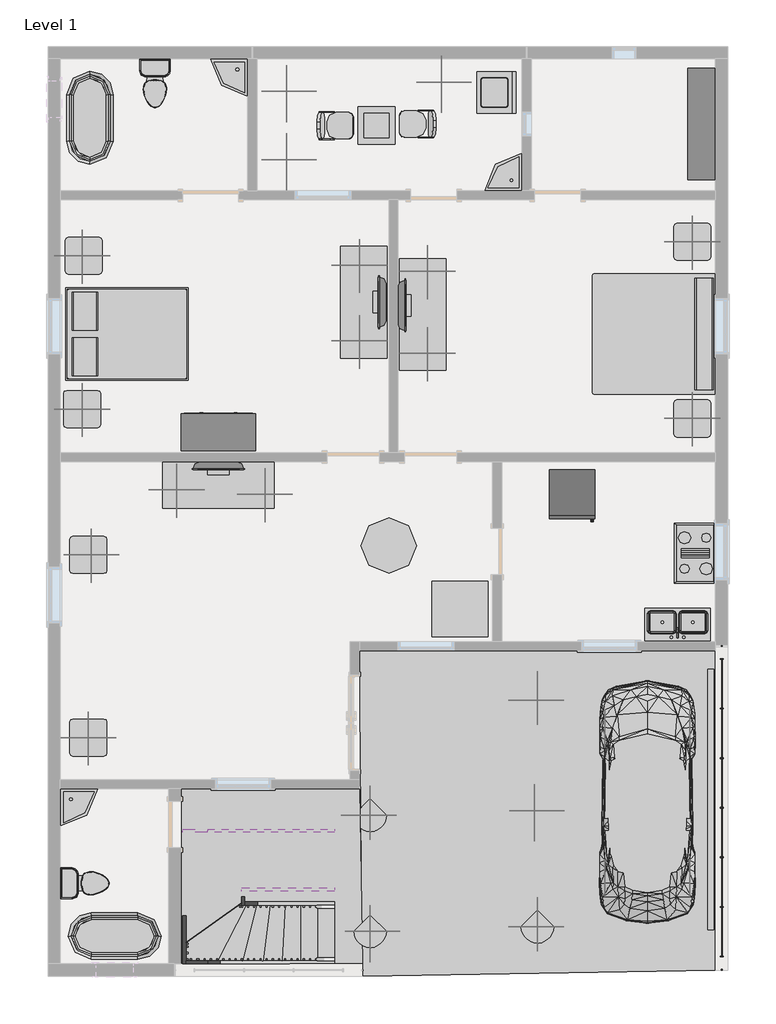
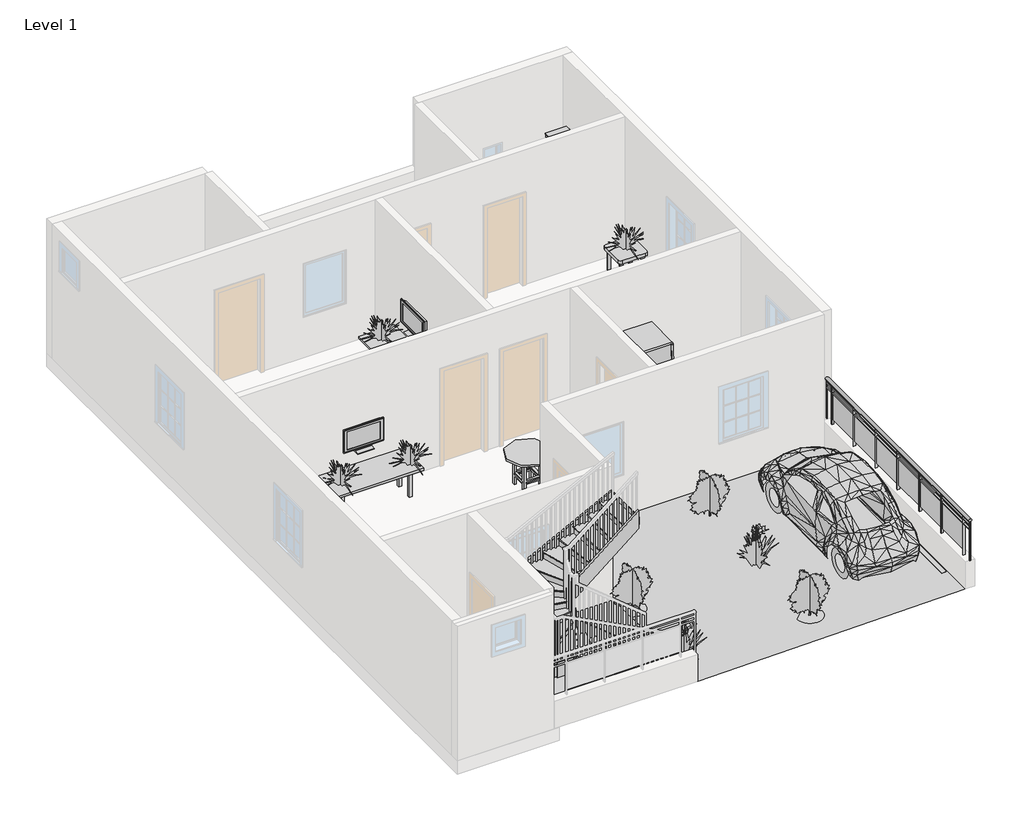
# One storey, part 3 of 3: 21 furniture elements, 20 geographic elements, 11 flow terminals, 8 members, 7 proxies, 1 railing, 1 stair flight.
"""IFC4 building model written with IfcOpenShell, lengths in millimetres."""

from ifc_helpers import new_model, si_unit, point, frame, origin, place, context, project, spatial, polyline, ellipse_curve, trimmed, outline, extrude, triangles, transform, mapped, element, save
from ifc_brep_helpers import plane_surface, extruded_surface, advanced_brep
from components import proxy_bb1e6e30, parking_space_9_x_18_90_deg_fdd9e8f5, rpc_beetle_rpc_beetle_3ce7ba48, proxy_a13a33b2, proxy_718fa39f, flow_terminal_accce45a, flow_terminal_bd5cdcf8, flow_terminal_a53be723, toilet_domestic_3d_toilet_domestic_3d_f7549cf7, toilet_domestic_3d_toilet_domestic_3d_183bbd19, flow_terminal_b374fae2, furniture_1d2926bd, furniture_1fc5af50, furniture_2babcf72, furniture_7c473f12, furniture_3d1d9cbc, furniture_56245f3a, furniture_b5c51a22, furniture_905aceb5, furniture_31d08a24, furniture_4d44e21c, furniture_62ce4b1f, rpc_plant_tropical_55f6ff97, rpc_plant_tropical_agave_1_5_93a2a214, rpc_plant_tropical_jungle_flame_3_9c4808c2, stair_flight_48a9080d

model = new_model("IFC4")

# Units and contexts
model_context = context("Model", 3, world=origin())
ifc_project = project(units=[si_unit("LENGTHUNIT", "METRE", prefix="MILLI")], contexts=[model_context])

# Site, building, storey
site = spatial("IfcSite", under=ifc_project)
building = spatial("IfcBuilding", under=site)
storey = spatial("IfcBuildingStorey", under=building, Name="Level 1", Elevation=0.0)

# Proxies
placement = place(None, origin())
element("IfcBuildingElementProxy", 1, Name="Building Element Proxy", at=placement, inside=storey, context=model_context, shape_type="Tessellation", body=[
    triangles([(-12555.3487518, 2203.3535912, 0.0), (-12555.3487518, -666.8463604, 0.0), (-7602.3493332, -666.8463604, 0.0), (-7653.1491394, 2203.3535912, 0.0)], [[1, 2, 4], [3, 4, 2]], closed=False),
])
element("IfcBuildingElementProxy", 2, Name="Building Element Proxy", at=placement, inside=storey, context=model_context, shape_type="Tessellation", body=[
    triangles([(-7653.1491394, 4463.953688, 0.0), (-7602.3493332, -870.0463846, 0.0), (-1811.1493332, -768.4463362, 0.0), (-1811.1493332, 4463.953688, 0.0)], [[1, 2, 3], [3, 4, 1]], closed=False),
])
proxy_shape = proxy_bb1e6e30(model_context)
element("IfcBuildingElementProxy", 3, Name="Cook Top-4 Unit : 36\" x 20\"", ObjectType="Cook Top-4 Unit : 36\" x 20\"", at=placement, inside=storey, context=model_context, shape_type="MappedRepresentation", body=[
    mapped(proxy_shape, transform((-2141.3492777, 6064.153629, 0.0), x_axis=(0.0, -1.0000000000000004, 0.0), y_axis=(1.0000000000000004, 0.0, 0.0), z_axis=(0.0, 0.0, 1.0))),
])
parking_space_9_x_18_90_deg_shape = parking_space_9_x_18_90_deg_fdd9e8f5(model_context)
element("IfcBuildingElementProxy", 4, Name="Parking Space : 9' x 18' - 90 deg", ObjectType="Parking Space : 9' x 18' - 90 deg", at=placement, inside=storey, context=model_context, shape_type="MappedRepresentation", body=[
    mapped(parking_space_9_x_18_90_deg_shape, transform((-1887.3492777, -108.046371, 0.0), x_axis=(-1.0, 0.0, 0.0), y_axis=(0.0, -1.0, 0.0), z_axis=(0.0, 0.0, 1.0))),
])
rpc_beetle_rpc_beetle_shape = rpc_beetle_rpc_beetle_3ce7ba48(model_context)
element("IfcBuildingElementProxy", 5, Name="RPC Beetle : RPC Beetle", ObjectType="RPC Beetle : RPC Beetle", at=placement, inside=storey, context=model_context, shape_type="MappedRepresentation", body=[
    mapped(rpc_beetle_rpc_beetle_shape, transform((-2928.7492777, 755.553629, 0.0), x_axis=(1.0, 0.0, 0.0), y_axis=(0.0, 1.0, 0.0), z_axis=(0.0, 0.0, 1.0))),
])
proxy_2_shape = proxy_a13a33b2(model_context)
element("IfcBuildingElementProxy", 6, Name="Refrigerator : 30\" x 32\" RH", ObjectType="Refrigerator : 30\" x 32\" RH", at=placement, inside=storey, context=model_context, shape_type="MappedRepresentation", body=[
    mapped(proxy_2_shape, transform((-4165.4117777, 7047.2046575, 0.0), x_axis=(1.0, 0.0, 0.0), y_axis=(0.0, 1.0, 0.0), z_axis=(0.0, 0.0, 1.0))),
])
proxy_3_shape = proxy_718fa39f(model_context)
element("IfcBuildingElementProxy", 7, Name="Washer : 27\" x 25\" x 35\"", ObjectType="Washer : 27\" x 25\" x 35\"", at=placement, inside=storey, context=model_context, shape_type="MappedRepresentation", body=[
    mapped(proxy_3_shape, transform((-5684.8997129, 14038.4361605, 0.0), x_axis=(0.0, -1.0000000000000004, 0.0), y_axis=(1.0000000000000004, 0.0, 0.0), z_axis=(0.0, 0.0, 1.0))),
])

# Flow terminals
flow_terminal_shape = flow_terminal_accce45a(model_context)
element("IfcFlowTerminal", 8, ObjectType="Floor Drain - Round : 5\" Strainer - 2\" Drain", at=placement, inside=storey, context=model_context, shape_type="MappedRepresentation", body=[
    mapped(flow_terminal_shape, transform((-11437.7492777, 12439.553629, 0.0), x_axis=(1.0, 0.0, 0.0), y_axis=(0.0, 1.0, 0.0), z_axis=(0.0, 0.0, 1.0))),
])
element("IfcFlowTerminal", 9, ObjectType="Floor Drain - Round : 5\" Strainer - 2\" Drain", at=placement, inside=storey, context=model_context, shape_type="MappedRepresentation", body=[
    mapped(flow_terminal_shape, transform((-5214.7492777, 12922.153629, 0.0), x_axis=(1.0, 0.0, 0.0), y_axis=(0.0, 1.0, 0.0), z_axis=(0.0, 0.0, 1.0))),
])
element("IfcFlowTerminal", 10, ObjectType="Floor Drain - Round : 5\" Strainer - 2\" Drain", at=placement, inside=storey, context=model_context, shape_type="MappedRepresentation", body=[
    mapped(flow_terminal_shape, transform((-11031.3492777, 425.353629, 0.0), x_axis=(1.0, 0.0, 0.0), y_axis=(0.0, 1.0, 0.0), z_axis=(0.0, 0.0, 1.0))),
])
flow_terminal_2_shape = flow_terminal_bd5cdcf8(model_context)
element("IfcFlowTerminal", 11, ObjectType="Sink - Corner Floor : 24\"", at=placement, inside=storey, context=model_context, shape_type="MappedRepresentation", body=[
    mapped(flow_terminal_2_shape, transform((-9481.9492777, 14166.753629, 914.4), x_axis=(-0.9999999999999998, 0.0, 0.0), y_axis=(0.0, -0.9999999999999998, 0.0), z_axis=(0.0, 0.0, 1.0))),
])
element("IfcFlowTerminal", 12, ObjectType="Sink - Corner Floor : 24\"", at=placement, inside=storey, context=model_context, shape_type="MappedRepresentation", body=[
    mapped(flow_terminal_2_shape, transform((-4986.1492777, 12007.753629, 914.4), x_axis=(0.0, 1.0, 0.0), y_axis=(-1.0, 0.0, 0.0), z_axis=(0.0, 0.0, 1.0))),
])
element("IfcFlowTerminal", 13, ObjectType="Sink - Corner Floor : 24\"", at=placement, inside=storey, context=model_context, shape_type="MappedRepresentation", body=[
    mapped(flow_terminal_2_shape, transform((-12555.3492777, 2203.353629, 914.4), x_axis=(0.0, -1.0000000000000004, 0.0), y_axis=(1.0000000000000004, 0.0, 0.0), z_axis=(0.0, 0.0, 1.0))),
])
flow_terminal_3_shape = flow_terminal_a53be723(model_context)
element("IfcFlowTerminal", 14, ObjectType="Sink Kitchen-Double : 42\" x 21\"", at=placement, inside=storey, context=model_context, shape_type="MappedRepresentation", body=[
    mapped(flow_terminal_3_shape, transform((-2417.7600371, 4898.0990301, 0.0), x_axis=(-1.0000000000000004, 0.0, 0.0), y_axis=(0.0, -1.0000000000000004, 0.0), z_axis=(0.0, 0.0, 1.0))),
])
toilet_domestic_3d_toilet_domestic_3d_shape = toilet_domestic_3d_toilet_domestic_3d_f7549cf7(model_context)
toilet_domestic_3d_toilet_domestic_3d_2_shape = toilet_domestic_3d_toilet_domestic_3d_183bbd19(model_context)
element("IfcFlowTerminal", 15, ObjectType="Toilet-Domestic-3D : Toilet-Domestic-3D", at=placement, inside=storey, context=model_context, shape_type="MappedRepresentation", body=[
    mapped(toilet_domestic_3d_toilet_domestic_3d_shape, transform((-11005.9492777, 13672.0576017, 0.0), x_axis=(1.0, 0.0, 0.0), y_axis=(0.0, 1.0, 0.0), z_axis=(0.0, 0.0, 1.0))),
    mapped(toilet_domestic_3d_toilet_domestic_3d_2_shape, transform((-11005.9492777, 13672.0576017, 0.0), x_axis=(1.0, 0.0, 0.0), y_axis=(0.0, 1.0, 0.0), z_axis=(0.0, 0.0, 1.0))),
])
element("IfcFlowTerminal", 16, ObjectType="Toilet-Domestic-3D : Toilet-Domestic-3D", at=placement, inside=storey, context=model_context, shape_type="MappedRepresentation", body=[
    mapped(toilet_domestic_3d_toilet_domestic_3d_shape, transform((-12060.6532503, 653.953629, 0.0), x_axis=(0.0, 1.0000000000000004, 0.0), y_axis=(-1.0000000000000004, 0.0, 0.0), z_axis=(0.0, 0.0, 1.0))),
    mapped(toilet_domestic_3d_toilet_domestic_3d_2_shape, transform((-12060.6532503, 653.953629, 0.0), x_axis=(0.0, 1.0000000000000004, 0.0), y_axis=(-1.0000000000000004, 0.0, 0.0), z_axis=(0.0, 0.0, 1.0))),
])
flow_terminal_4_shape = flow_terminal_b374fae2(model_context)
element("IfcFlowTerminal", 17, ObjectType="Tub-Free Standing-3D : 30\" x 60\"", at=placement, inside=storey, context=model_context, shape_type="MappedRepresentation", body=[
    mapped(flow_terminal_4_shape, transform((-12072.7492777, 13201.553629, 0.0), x_axis=(-1.0000000000000004, 0.0, 0.0), y_axis=(0.0, -1.0000000000000004, 0.0), z_axis=(0.0, 0.0, 1.0))),
])
element("IfcFlowTerminal", 18, ObjectType="Tub-Free Standing-3D : 30\" x 60\"", at=placement, inside=storey, context=model_context, shape_type="MappedRepresentation", body=[
    mapped(flow_terminal_4_shape, transform((-11666.3492777, -209.646371, 0.0), x_axis=(0.0, 1.0, 0.0), y_axis=(-1.0, 0.0, 0.0), z_axis=(0.0, 0.0, 1.0))),
])

# Furniture
furniture_shape = furniture_1d2926bd(model_context)
element("IfcFurniture", 19, ObjectType="Bed-Box : Queen 60\" x 79\"", at=placement, inside=storey, context=model_context, shape_type="MappedRepresentation", body=[
    mapped(furniture_shape, transform((-11697.5787859, 9319.10117, 0.0), x_axis=(0.0, 1.0000000000000002, 0.0), y_axis=(-1.0000000000000002, 0.0, 0.0), z_axis=(0.0, 0.0, 1.0))),
])
furniture_2_shape = furniture_1fc5af50(model_context)
element("IfcFurniture", 20, ObjectType="Bed-Standard.0001 : King 78\" x 80\"", at=placement, inside=storey, context=model_context, shape_type="MappedRepresentation", body=[
    mapped(furniture_2_shape, transform((-2768.8541957, 9929.7421536, 0.0), x_axis=(0.0, -1.0, 0.0), y_axis=(1.0, 0.0, 0.0), z_axis=(0.0, 0.0, 1.0))),
])
furniture_3_shape = furniture_2babcf72(model_context)
element("IfcFurniture", 21, ObjectType="Dresser : 48\" x 60\" x 24\"", at=placement, inside=storey, context=model_context, shape_type="MappedRepresentation", body=[
    mapped(furniture_3_shape, transform((-10233.7425375, 7682.1906749, 0.0), x_axis=(-1.0000000000000004, 0.0, 0.0), y_axis=(0.0, -1.0000000000000004, 0.0), z_axis=(0.0, 0.0, 1.0))),
])
furniture_4_shape = furniture_7c473f12(model_context)
element("IfcFurniture", 22, ObjectType="Dresser : 72\" x 60\" x 18\"", at=placement, inside=storey, context=model_context, shape_type="MappedRepresentation", body=[
    mapped(furniture_4_shape, transform((-2402.9122318, 13369.1468889, 0.0), x_axis=(0.0, 1.0, 0.0), y_axis=(-1.0, 0.0, 0.0), z_axis=(0.0, 0.0, 1.0))),
])
furniture_5_shape = furniture_3d1d9cbc(model_context)
element("IfcFurniture", 23, ObjectType="Seating-Auditorium : 18\" x 24\" x 30\"", at=placement, inside=storey, context=model_context, shape_type="MappedRepresentation", body=[
    mapped(furniture_5_shape, transform((-6498.0738678, 12939.2257602, 0.0), x_axis=(0.0, 1.0, 0.0), y_axis=(-1.0, 0.0, 0.0), z_axis=(0.0, 0.0, 1.0))),
])
element("IfcFurniture", 24, ObjectType="Seating-Auditorium : 18\" x 24\" x 30\"", at=placement, inside=storey, context=model_context, shape_type="MappedRepresentation", body=[
    mapped(furniture_5_shape, transform((-8249.4246875, 13235.2814979, 0.0), x_axis=(0.0, -1.0000000000000004, 0.0), y_axis=(1.0000000000000004, 0.0, 0.0), z_axis=(0.0, 0.0, 1.0))),
])
furniture_6_shape = furniture_56245f3a(model_context)
element("IfcFurniture", 25, ObjectType="TV - Flat Screen : 32\"", at=placement, inside=storey, context=model_context, shape_type="MappedRepresentation", body=[
    mapped(furniture_6_shape, transform((-7273.5379013, 10175.0091149, 1041.4), x_axis=(0.0, -1.0000000000000004, 0.0), y_axis=(1.0000000000000004, 0.0, 0.0), z_axis=(0.0, 0.0, 1.0))),
])
element("IfcFurniture", 26, ObjectType="TV - Flat Screen : 32\"", at=placement, inside=storey, context=model_context, shape_type="MappedRepresentation", body=[
    mapped(furniture_6_shape, transform((-6959.610654, 10132.0981432, 1041.4), x_axis=(0.0, 1.0, 0.0), y_axis=(-1.0, 0.0, 0.0), z_axis=(0.0, 0.0, 1.0))),
])
element("IfcFurniture", 27, ObjectType="TV - Flat Screen : 32\"", at=placement, inside=storey, context=model_context, shape_type="MappedRepresentation", body=[
    mapped(furniture_6_shape, transform((-9960.6047635, 7504.2150054, 1041.4), x_axis=(1.0, 0.0, 0.0), y_axis=(0.0, 1.0, 0.0), z_axis=(0.0, 0.0, 1.0))),
])
furniture_7_shape = furniture_b5c51a22(model_context)
element("IfcFurniture", 28, ObjectType="Table-Coffee : 24\" x 24\" x 24\"", at=placement, inside=storey, context=model_context, shape_type="MappedRepresentation", body=[
    mapped(furniture_7_shape, transform((-7392.0150443, 12979.3425512, 0.0), x_axis=(1.0, 0.0, 0.0), y_axis=(0.0, 1.0, 0.0), z_axis=(0.0, 0.0, 1.0))),
])
furniture_8_shape = furniture_905aceb5(model_context)
element("IfcFurniture", 29, ObjectType="Table-Dining Round w Chairs : 36\" Diameter", at=placement, inside=storey, context=model_context, shape_type="MappedRepresentation", body=[
    mapped(furniture_8_shape, transform((-7274.2312449, 6376.0323176, 0.0), x_axis=(1.0, 0.0, 0.0), y_axis=(0.0, 1.0, 0.0), z_axis=(0.0, 0.0, 1.0))),
])
furniture_9_shape = furniture_31d08a24(model_context)
element("IfcFurniture", 30, ObjectType="Table-End : 24\" x 24\"", at=placement, inside=storey, context=model_context, shape_type="MappedRepresentation", body=[
    mapped(furniture_9_shape, transform((-12482.8829079, 10788.553629, 0.0), x_axis=(1.0, 0.0, 0.0), y_axis=(0.0, 1.0, 0.0), z_axis=(0.0, 0.0, 1.0))),
])
element("IfcFurniture", 31, ObjectType="Table-End : 24\" x 24\"", at=placement, inside=storey, context=model_context, shape_type="MappedRepresentation", body=[
    mapped(furniture_9_shape, transform((-12508.2829079, 8273.953629, 0.0), x_axis=(1.0, 0.0, 0.0), y_axis=(0.0, 1.0, 0.0), z_axis=(0.0, 0.0, 1.0))),
])
element("IfcFurniture", 32, ObjectType="Table-End : 24\" x 24\"", at=placement, inside=storey, context=model_context, shape_type="MappedRepresentation", body=[
    mapped(furniture_9_shape, transform((-2500.6829079, 11017.153629, 0.0), x_axis=(1.0, 0.0, 0.0), y_axis=(0.0, 1.0, 0.0), z_axis=(0.0, 0.0, 1.0))),
])
element("IfcFurniture", 33, ObjectType="Table-End : 24\" x 24\"", at=placement, inside=storey, context=model_context, shape_type="MappedRepresentation", body=[
    mapped(furniture_9_shape, transform((-2500.6829079, 8121.553629, 0.0), x_axis=(1.0, 0.0, 0.0), y_axis=(0.0, 1.0, 0.0), z_axis=(0.0, 0.0, 1.0))),
])
element("IfcFurniture", 34, ObjectType="Table-End : 24\" x 24\"", at=placement, inside=storey, context=model_context, shape_type="MappedRepresentation", body=[
    mapped(furniture_9_shape, transform((-12406.6829079, 2889.153629, 0.0), x_axis=(1.0, 0.0, 0.0), y_axis=(0.0, 1.0, 0.0), z_axis=(0.0, 0.0, 1.0))),
])
element("IfcFurniture", 35, ObjectType="Table-End : 24\" x 24\"", at=placement, inside=storey, context=model_context, shape_type="MappedRepresentation", body=[
    mapped(furniture_9_shape, transform((-12406.6829079, 5886.353629, 0.0), x_axis=(1.0, 0.0, 0.0), y_axis=(0.0, 1.0, 0.0), z_axis=(0.0, 0.0, 1.0))),
])
furniture_10_shape = furniture_4d44e21c(model_context)
element("IfcFurniture", 36, ObjectType="Table-Rectangular : 36\" x 36\"", at=placement, inside=storey, context=model_context, shape_type="MappedRepresentation", body=[
    mapped(furniture_10_shape, transform((-6002.1492777, 5149.753629, 0.0), x_axis=(0.0, 1.0000000000000002, 0.0), y_axis=(-1.0000000000000002, 0.0, 0.0), z_axis=(0.0, 0.0, 1.0))),
])
furniture_11_shape = furniture_62ce4b1f(model_context)
element("IfcFurniture", 37, ObjectType="Table-Rectangular : 72\" x 30\"", at=placement, inside=storey, context=model_context, shape_type="MappedRepresentation", body=[
    mapped(furniture_11_shape, transform((-7576.9492777, 10178.953629, 0.0), x_axis=(0.0, 1.0000000000000002, 0.0), y_axis=(-1.0000000000000002, 0.0, 0.0), z_axis=(0.0, 0.0, 1.0))),
])
element("IfcFurniture", 38, ObjectType="Table-Rectangular : 72\" x 30\"", at=placement, inside=storey, context=model_context, shape_type="MappedRepresentation", body=[
    mapped(furniture_11_shape, transform((-6611.7492777, 9975.753629, 0.0), x_axis=(0.0, 1.0000000000000002, 0.0), y_axis=(-1.0000000000000002, 0.0, 0.0), z_axis=(0.0, 0.0, 1.0))),
])
element("IfcFurniture", 39, ObjectType="Table-Rectangular : 72\" x 30\"", at=placement, inside=storey, context=model_context, shape_type="MappedRepresentation", body=[
    mapped(furniture_11_shape, transform((-9964.5492777, 7181.753629, 0.0), x_axis=(1.0, 0.0, 0.0), y_axis=(0.0, 1.0, 0.0), z_axis=(0.0, 0.0, 1.0))),
])

# Geographic elements
rpc_plant_tropical_shape = rpc_plant_tropical_55f6ff97(model_context)
element("IfcGeographicElement", 40, ObjectType="RPC Plant - Tropical", at=placement, inside=storey, context=model_context, shape_type="MappedRepresentation", body=[
    mapped(rpc_plant_tropical_shape, transform((-8846.9492777, 13633.353629, 0.0), x_axis=(1.0, 0.0, 0.0), y_axis=(0.0, 1.0, 0.0), z_axis=(0.0, 0.0, 1.0))),
])
element("IfcGeographicElement", 41, ObjectType="RPC Plant - Tropical", at=placement, inside=storey, context=model_context, shape_type="MappedRepresentation", body=[
    mapped(rpc_plant_tropical_shape, transform((-8846.9492777, 12515.753629, 0.0), x_axis=(1.0, 0.0, 0.0), y_axis=(0.0, 1.0, 0.0), z_axis=(0.0, 0.0, 1.0))),
])
element("IfcGeographicElement", 42, ObjectType="RPC Plant - Tropical", at=placement, inside=storey, context=model_context, shape_type="MappedRepresentation", body=[
    mapped(rpc_plant_tropical_shape, transform((-6306.9492777, 13785.753629, 0.0), x_axis=(1.0, 0.0, 0.0), y_axis=(0.0, 1.0, 0.0), z_axis=(0.0, 0.0, 1.0))),
])
element("IfcGeographicElement", 43, ObjectType="RPC Plant - Tropical", at=placement, inside=storey, context=model_context, shape_type="MappedRepresentation", body=[
    mapped(rpc_plant_tropical_shape, transform((-4782.9492777, 1847.753629, 0.0), x_axis=(1.0, 0.0, 0.0), y_axis=(0.0, 1.0, 0.0), z_axis=(0.0, 0.0, 1.0))),
])
element("IfcGeographicElement", 44, ObjectType="RPC Plant - Tropical", at=placement, inside=storey, context=model_context, shape_type="MappedRepresentation", body=[
    mapped(rpc_plant_tropical_shape, transform((-7475.3492777, -133.446371, 0.0), x_axis=(1.0, 0.0, 0.0), y_axis=(0.0, 1.0, 0.0), z_axis=(0.0, 0.0, 1.0))),
])
rpc_plant_tropical_agave_1_5_shape = rpc_plant_tropical_agave_1_5_93a2a214(model_context)
element("IfcGeographicElement", 45, ObjectType="RPC Plant - Tropical : Agave - 1.5'", at=placement, inside=storey, context=model_context, shape_type="MappedRepresentation", body=[
    mapped(rpc_plant_tropical_agave_1_5_shape, transform((-12199.7492777, 10940.953629, 609.6), x_axis=(1.0, 0.0, 0.0), y_axis=(0.0, 1.0, 0.0), z_axis=(0.0, 0.0, 1.0))),
])
element("IfcGeographicElement", 46, ObjectType="RPC Plant - Tropical : Agave - 1.5'", at=placement, inside=storey, context=model_context, shape_type="MappedRepresentation", body=[
    mapped(rpc_plant_tropical_agave_1_5_shape, transform((-12199.7492777, 8426.353629, 609.6), x_axis=(1.0, 0.0, 0.0), y_axis=(0.0, 1.0, 0.0), z_axis=(0.0, 0.0, 1.0))),
])
element("IfcGeographicElement", 47, ObjectType="RPC Plant - Tropical : Agave - 1.5'", at=placement, inside=storey, context=model_context, shape_type="MappedRepresentation", body=[
    mapped(rpc_plant_tropical_agave_1_5_shape, transform((-7653.1492777, 10788.553629, 685.8), x_axis=(1.0, 0.0, 0.0), y_axis=(0.0, 1.0, 0.0), z_axis=(0.0, 0.0, 1.0))),
])
element("IfcGeographicElement", 48, ObjectType="RPC Plant - Tropical : Agave - 1.5'", at=placement, inside=storey, context=model_context, shape_type="MappedRepresentation", body=[
    mapped(rpc_plant_tropical_agave_1_5_shape, transform((-7653.1492777, 9543.953629, 685.8), x_axis=(1.0, 0.0, 0.0), y_axis=(0.0, 1.0, 0.0), z_axis=(0.0, 0.0, 1.0))),
])
element("IfcGeographicElement", 49, ObjectType="RPC Plant - Tropical : Agave - 1.5'", at=placement, inside=storey, context=model_context, shape_type="MappedRepresentation", body=[
    mapped(rpc_plant_tropical_agave_1_5_shape, transform((-2192.1492777, 11169.553629, 609.6), x_axis=(1.0, 0.0, 0.0), y_axis=(0.0, 1.0, 0.0), z_axis=(0.0, 0.0, 1.0))),
])
element("IfcGeographicElement", 50, ObjectType="RPC Plant - Tropical : Agave - 1.5'", at=placement, inside=storey, context=model_context, shape_type="MappedRepresentation", body=[
    mapped(rpc_plant_tropical_agave_1_5_shape, transform((-2192.1492777, 8273.953629, 609.6), x_axis=(1.0, 0.0, 0.0), y_axis=(0.0, 1.0, 0.0), z_axis=(0.0, 0.0, 1.0))),
])
element("IfcGeographicElement", 51, ObjectType="RPC Plant - Tropical : Agave - 1.5'", at=placement, inside=storey, context=model_context, shape_type="MappedRepresentation", body=[
    mapped(rpc_plant_tropical_agave_1_5_shape, transform((-6535.5492777, 10686.953629, 685.8), x_axis=(1.0, 0.0, 0.0), y_axis=(0.0, 1.0, 0.0), z_axis=(0.0, 0.0, 1.0))),
])
element("IfcGeographicElement", 52, ObjectType="RPC Plant - Tropical : Agave - 1.5'", at=placement, inside=storey, context=model_context, shape_type="MappedRepresentation", body=[
    mapped(rpc_plant_tropical_agave_1_5_shape, transform((-6535.5492777, 9340.753629, 685.8), x_axis=(1.0, 0.0, 0.0), y_axis=(0.0, 1.0, 0.0), z_axis=(0.0, 0.0, 1.0))),
])
element("IfcGeographicElement", 53, ObjectType="RPC Plant - Tropical : Agave - 1.5'", at=placement, inside=storey, context=model_context, shape_type="MappedRepresentation", body=[
    mapped(rpc_plant_tropical_agave_1_5_shape, transform((-12047.3492777, 6038.753629, 609.6), x_axis=(1.0, 0.0, 0.0), y_axis=(0.0, 1.0, 0.0), z_axis=(0.0, 0.0, 1.0))),
])
element("IfcGeographicElement", 54, ObjectType="RPC Plant - Tropical : Agave - 1.5'", at=placement, inside=storey, context=model_context, shape_type="MappedRepresentation", body=[
    mapped(rpc_plant_tropical_agave_1_5_shape, transform((-12098.1492777, 3041.553629, 609.6), x_axis=(1.0, 0.0, 0.0), y_axis=(0.0, 1.0, 0.0), z_axis=(0.0, 0.0, 1.0))),
])
element("IfcGeographicElement", 55, ObjectType="RPC Plant - Tropical : Agave - 1.5'", at=placement, inside=storey, context=model_context, shape_type="MappedRepresentation", body=[
    mapped(rpc_plant_tropical_agave_1_5_shape, transform((-9202.5492777, 7029.353629, 685.8), x_axis=(1.0, 0.0, 0.0), y_axis=(0.0, 1.0, 0.0), z_axis=(0.0, 0.0, 1.0))),
])
element("IfcGeographicElement", 56, ObjectType="RPC Plant - Tropical : Agave - 1.5'", at=placement, inside=storey, context=model_context, shape_type="MappedRepresentation", body=[
    mapped(rpc_plant_tropical_agave_1_5_shape, transform((-10650.3492777, 7105.553629, 685.8), x_axis=(1.0, 0.0, 0.0), y_axis=(0.0, 1.0, 0.0), z_axis=(0.0, 0.0, 1.0))),
])
rpc_plant_tropical_jungle_flame_3_shape = rpc_plant_tropical_jungle_flame_3_9c4808c2(model_context)
element("IfcGeographicElement", 57, ObjectType="RPC Plant - Tropical : Jungle Flame - 3'", at=placement, inside=storey, context=model_context, shape_type="MappedRepresentation", body=[
    mapped(rpc_plant_tropical_jungle_flame_3_shape, transform((-4732.1492777, -57.246371, 0.0), x_axis=(1.0, 0.0, 0.0), y_axis=(0.0, 1.0, 0.0), z_axis=(0.0, 0.0, 1.0))),
])
element("IfcGeographicElement", 58, ObjectType="RPC Plant - Tropical : Jungle Flame - 3'", at=placement, inside=storey, context=model_context, shape_type="MappedRepresentation", body=[
    mapped(rpc_plant_tropical_jungle_flame_3_shape, transform((-7475.3492777, 1771.553629, 0.0), x_axis=(1.0, 0.0, 0.0), y_axis=(0.0, 1.0, 0.0), z_axis=(0.0, 0.0, 1.0))),
])
element("IfcGeographicElement", 59, ObjectType="RPC Plant - Tropical : Jungle Flame - 3'", at=placement, inside=storey, context=model_context, shape_type="MappedRepresentation", body=[
    mapped(rpc_plant_tropical_jungle_flame_3_shape, transform((-4732.1492777, 3651.153629, 0.0), x_axis=(1.0, 0.0, 0.0), y_axis=(0.0, 1.0, 0.0), z_axis=(0.0, 0.0, 1.0))),
])

# Members
element("IfcMember", 60, ObjectType="Stringer - 2\" Width", at=placement, inside=storey, context=model_context, shape_type="SweptSolid", body=[
    extrude(outline(polyline([(0.0, -8055.8175858), (229.639954, -8055.8175858), (1305.3956453, -10143.2347775), (962.500629, -10143.2347775), (0.0, -8275.5799034), (0.0, -8055.8175858)])), frame((0.0, -666.846371, 0.0), z_axis=(0.0, 1.0, 0.0), x_axis=(0.0, 0.0, 1.0)), (0.0, 0.0, 1.0), 50.8),
])
element("IfcMember", 61, ObjectType="Stringer - 2\" Width", at=placement, inside=storey, context=model_context, shape_type="SweptSolid", body=[
    extrude(outline(polyline([(-10143.2347775, -616.046371), (-10143.2347775, -666.846371), (-10497.9492777, -666.846371), (-10497.9492777, -616.046371), (-10143.2347775, -616.046371)])), frame((0.0, 0.0, 962.500629), z_axis=(0.0, 0.0, 1.0), x_axis=(1.0, 0.0, 0.0)), (0.0, 0.0, 1.0), 342.8950162),
])
element("IfcMember", 62, ObjectType="Stringer - 2\" Width", at=placement, inside=storey, context=model_context, shape_type="SweptSolid", body=[
    extrude(outline(polyline([(-666.846371, 1000.5956453), (-666.846371, 1289.0952212), (1455.1735117, 1969.9972697), (1492.153629, 1969.9972697), (1492.153629, 1638.9682298), (-497.323888, 1000.5956453), (-666.846371, 1000.5956453)])), frame((-10548.7492777, 0.0, 0.0), z_axis=(1.0, 0.0, 0.0), x_axis=(0.0, 1.0, 0.0)), (0.0, 0.0, 1.0), 50.8),
])
element("IfcMember", 63, ObjectType="Stringer - 2\" Width", at=placement, inside=storey, context=model_context, shape_type="SweptSolid", body=[
    extrude(outline(polyline([(-10548.7492777, 1492.153629), (-10548.7492777, 1542.953629), (-10143.2347775, 1542.953629), (-10143.2347775, 1492.153629), (-10548.7492777, 1492.153629)])), frame((0.0, 0.0, 1649.8904473), z_axis=(0.0, 0.0, 1.0), x_axis=(1.0, 0.0, 0.0)), (0.0, 0.0, 1.0), 320.1068224),
])
element("IfcMember", 64, ObjectType="Stringer - 2\" Width", at=placement, inside=storey, context=model_context, shape_type="SweptSolid", body=[
    extrude(outline(polyline([(1969.9972697, -10143.2347775), (1649.8904473, -10143.2347775), (2725.6461385, -8055.8175858), (3045.7529609, -8055.8175858), (1969.9972697, -10143.2347775)])), frame((0.0, 1492.153629, 0.0), z_axis=(0.0, 1.0, 0.0), x_axis=(0.0, 0.0, 1.0)), (0.0, 0.0, 1.0), 50.8),
])
element("IfcMember", 65, ObjectType="Stringer - 2\" Width", at=placement, inside=storey, context=model_context, shape_type="SweptSolid", body=[
    extrude(outline(polyline([(0.0, -8055.8175858), (176.1764461, -8055.8175858), (1380.418648, -9532.7492777), (987.1410923, -9532.7492777), (0.0, -8322.0792303), (0.0, -8055.8175858)])), frame((0.0, 298.353629, 0.0), z_axis=(0.0, 1.0, 0.0), x_axis=(0.0, 0.0, 1.0)), (0.0, 0.0, 1.0), 50.8),
])
element("IfcMember", 66, ObjectType="Stringer - 2\" Width", at=placement, inside=storey, context=model_context, shape_type="SweptSolid", body=[
    extrude(outline(polyline([(298.353629, 1028.5617647), (298.353629, 1573.2682978), (504.9907465, 1926.1409689), (526.953629, 1926.1409689), (526.953629, 1360.465107), (332.5958463, 1028.5617647), (298.353629, 1028.5617647)])), frame((-9583.5492777, 0.0, 0.0), z_axis=(1.0, 0.0, 0.0), x_axis=(0.0, 1.0, 0.0)), (0.0, 0.0, 1.0), 50.8),
])
element("IfcMember", 67, ObjectType="Stringer - 2\" Width", at=placement, inside=storey, context=model_context, shape_type="SweptSolid", body=[
    extrude(outline(polyline([(1926.1409689, -9583.5492777), (1532.8634131, -9583.5492777), (2778.5262875, -8055.8175858), (3171.8038432, -8055.8175858), (1926.1409689, -9583.5492777)])), frame((0.0, 526.953629, 0.0), z_axis=(0.0, 1.0, 0.0), x_axis=(0.0, 0.0, 1.0)), (0.0, 0.0, 1.0), 50.8),
])

# Railing
element("IfcRailing", 68, ObjectType="Glass Panel - Bottom Fill", at=placement, inside=storey, context=model_context, shape_type="SolidModel", body=[
    advanced_brep(
    [(-1671.4492777, 4552.853629, 1524.0), (-1747.6492777, 4552.853629, 1524.0), (-1671.4492777, -768.446371, 1524.0), (-1747.6492777, -768.446371, 1524.0)],
    [
        (0, 1, ellipse_curve(frame((-1709.5492777, 4552.853629, 1524.0), z_axis=(0.0, 1.0, 0.0), x_axis=(-1.0, 0.0, 0.0)), 38.1, 28.575)),
        (1, 0, ellipse_curve(frame((-1709.5492777, 4552.853629, 1524.0), z_axis=(0.0, 1.0, 0.0), x_axis=(-1.0, 0.0, 0.0)), 38.1, 28.575)),
        (2, 3, ellipse_curve(frame((-1709.5492777, -768.446371, 1524.0), z_axis=(0.0, -1.0, 0.0), x_axis=(-1.0, 0.0, 0.0)), 38.1, 28.575)),
        (3, 2, ellipse_curve(frame((-1709.5492777, -768.446371, 1524.0), z_axis=(0.0, -1.0, 0.0), x_axis=(-1.0, 0.0, 0.0)), 38.1, 28.575)),
        (0, 2),
        (3, 1),
    ],
    [
        plane_surface(frame((-1709.5492777, 4552.853629, 1524.0), z_axis=(0.0, 1.0, 0.0), x_axis=(0.0, 0.0, -1.0))),
        plane_surface(frame((-1709.5492777, -768.446371, 1524.0), z_axis=(0.0, -1.0, 0.0), x_axis=(0.0, 0.0, -1.0))),
        extruded_surface(trimmed(ellipse_curve(frame((-1709.5492777, -768.446371, 1524.0), z_axis=(0.0, 1.0, 0.0), x_axis=(-1.0, 0.0, 0.0)), 38.1, 28.575), [point((-1671.4492777, -768.446371, 1524.0))], [point((-1747.6492777, -768.446371, 1524.0))], True, "CARTESIAN"), (0.0, 5321.3, 0.0), 5321.3),
        extruded_surface(trimmed(ellipse_curve(frame((-1709.5492777, -768.446371, 1524.0), z_axis=(0.0, 1.0, 0.0), x_axis=(-1.0, 0.0, 0.0)), 38.1, 28.575), [point((-1747.6492777, -768.446371, 1524.0))], [point((-1671.4492777, -768.446371, 1524.0))], True, "CARTESIAN"), (0.0, 5321.3, 0.0), 5321.3),
    ],
    [
        (0, [[1, 2]]),
        (1, [[3, 4]]),
        (2, [[-1, 5, -4, 6]]),
        (3, [[-2, -6, -3, -5]]),
    ],
),
    extrude(outline(polyline([(-1722.2492777, 4552.853629), (-1696.8492777, 4552.853629), (-1696.8492777, -768.446371), (-1722.2492777, -768.446371), (-1722.2492777, 4552.853629)])), frame((0.0, 0.0, 1409.7), z_axis=(0.0, 0.0, 1.0), x_axis=(1.0, 0.0, 0.0)), (0.0, 0.0, 1.0), 25.4),
    extrude(outline(polyline([(-1722.2492777, 4552.853629), (-1696.8492777, 4552.853629), (-1696.8492777, -768.446371), (-1722.2492777, -768.446371), (-1722.2492777, 4552.853629)])), frame((0.0, 0.0, 1308.1), z_axis=(0.0, 0.0, 1.0), x_axis=(1.0, 0.0, 0.0)), (0.0, 0.0, 1.0), 25.4),
    extrude(outline(polyline([(-1734.9492777, -539.846371), (-1684.1492777, -539.846371), (-1684.1492777, -552.546371), (-1734.9492777, -552.546371), (-1734.9492777, -539.846371)])), frame((0.0, 0.0, 609.6), z_axis=(0.0, 0.0, 1.0), x_axis=(1.0, 0.0, 0.0)), (0.0, 0.0, 1.0), 885.6788223),
    extrude(outline(polyline([(-1703.0141207, 266.603629), (-1703.0141207, -546.196371), (-1709.3641207, -546.196371), (-1709.3641207, 266.603629), (-1703.0141207, 266.603629)])), frame((0.0, 0.0, 711.2), z_axis=(0.0, 0.0, 1.0), x_axis=(1.0, 0.0, 0.0)), (0.0, 0.0, 1.0), 596.9),
    extrude(outline(polyline([(-1734.9492777, 272.953629), (-1684.1492777, 272.953629), (-1684.1492777, 260.253629), (-1734.9492777, 260.253629), (-1734.9492777, 272.953629)])), frame((0.0, 0.0, 609.6), z_axis=(0.0, 0.0, 1.0), x_axis=(1.0, 0.0, 0.0)), (0.0, 0.0, 1.0), 885.6788223),
    extrude(outline(polyline([(-1703.0141207, 1079.403629), (-1703.0141207, 266.603629), (-1709.3641207, 266.603629), (-1709.3641207, 1079.403629), (-1703.0141207, 1079.403629)])), frame((0.0, 0.0, 711.2), z_axis=(0.0, 0.0, 1.0), x_axis=(1.0, 0.0, 0.0)), (0.0, 0.0, 1.0), 596.9),
    extrude(outline(polyline([(-1734.9492777, 1085.753629), (-1684.1492777, 1085.753629), (-1684.1492777, 1073.053629), (-1734.9492777, 1073.053629), (-1734.9492777, 1085.753629)])), frame((0.0, 0.0, 609.6), z_axis=(0.0, 0.0, 1.0), x_axis=(1.0, 0.0, 0.0)), (0.0, 0.0, 1.0), 885.6788223),
    extrude(outline(polyline([(-1703.0141207, 1892.203629), (-1703.0141207, 1079.403629), (-1709.3641207, 1079.403629), (-1709.3641207, 1892.203629), (-1703.0141207, 1892.203629)])), frame((0.0, 0.0, 711.2), z_axis=(0.0, 0.0, 1.0), x_axis=(1.0, 0.0, 0.0)), (0.0, 0.0, 1.0), 596.9),
    extrude(outline(polyline([(-1734.9492777, 1898.553629), (-1684.1492777, 1898.553629), (-1684.1492777, 1885.853629), (-1734.9492777, 1885.853629), (-1734.9492777, 1898.553629)])), frame((0.0, 0.0, 609.6), z_axis=(0.0, 0.0, 1.0), x_axis=(1.0, 0.0, 0.0)), (0.0, 0.0, 1.0), 885.6788223),
    extrude(outline(polyline([(-1703.0141207, 2705.003629), (-1703.0141207, 1892.203629), (-1709.3641207, 1892.203629), (-1709.3641207, 2705.003629), (-1703.0141207, 2705.003629)])), frame((0.0, 0.0, 711.2), z_axis=(0.0, 0.0, 1.0), x_axis=(1.0, 0.0, 0.0)), (0.0, 0.0, 1.0), 596.9),
    extrude(outline(polyline([(-1734.9492777, 2711.353629), (-1684.1492777, 2711.353629), (-1684.1492777, 2698.653629), (-1734.9492777, 2698.653629), (-1734.9492777, 2711.353629)])), frame((0.0, 0.0, 609.6), z_axis=(0.0, 0.0, 1.0), x_axis=(1.0, 0.0, 0.0)), (0.0, 0.0, 1.0), 885.6788223),
    extrude(outline(polyline([(-1703.0141207, 3517.803629), (-1703.0141207, 2705.003629), (-1709.3641207, 2705.003629), (-1709.3641207, 3517.803629), (-1703.0141207, 3517.803629)])), frame((0.0, 0.0, 711.2), z_axis=(0.0, 0.0, 1.0), x_axis=(1.0, 0.0, 0.0)), (0.0, 0.0, 1.0), 596.9),
    extrude(outline(polyline([(-1734.9492777, 3524.153629), (-1684.1492777, 3524.153629), (-1684.1492777, 3511.453629), (-1734.9492777, 3511.453629), (-1734.9492777, 3524.153629)])), frame((0.0, 0.0, 609.6), z_axis=(0.0, 0.0, 1.0), x_axis=(1.0, 0.0, 0.0)), (0.0, 0.0, 1.0), 885.6788223),
    extrude(outline(polyline([(-1703.0141207, 4330.603629), (-1703.0141207, 3517.803629), (-1709.3641207, 3517.803629), (-1709.3641207, 4330.603629), (-1703.0141207, 4330.603629)])), frame((0.0, 0.0, 711.2), z_axis=(0.0, 0.0, 1.0), x_axis=(1.0, 0.0, 0.0)), (0.0, 0.0, 1.0), 596.9),
    extrude(outline(polyline([(-1734.9492777, 4336.953629), (-1684.1492777, 4336.953629), (-1684.1492777, 4324.253629), (-1734.9492777, 4324.253629), (-1734.9492777, 4336.953629)])), frame((0.0, 0.0, 609.6), z_axis=(0.0, 0.0, 1.0), x_axis=(1.0, 0.0, 0.0)), (0.0, 0.0, 1.0), 885.6788223),
    extrude(outline(polyline([(-1719.0742777, -755.746371), (-1700.0242777, -755.746371), (-1700.0242777, -774.796371), (-1719.0742777, -774.796371), (-1719.0742777, -755.746371)])), frame((0.0, 0.0, 609.6), z_axis=(0.0, 0.0, 1.0), x_axis=(1.0, 0.0, 0.0)), (0.0, 0.0, 1.0), 885.6788223),
    extrude(outline(polyline([(-1719.0742777, 4559.203629), (-1700.0242777, 4559.203629), (-1700.0242777, 4540.153629), (-1719.0742777, 4540.153629), (-1719.0742777, 4559.203629)])), frame((0.0, 0.0, 609.6), z_axis=(0.0, 0.0, 1.0), x_axis=(1.0, 0.0, 0.0)), (0.0, 0.0, 1.0), 885.6788223),
])

# Stair flight
stair_flight_shape = stair_flight_48a9080d(model_context)
element("IfcStairFlight", 69, ObjectType="2\" Tread 1\" Nosing 1/4\" Riser", at=placement, inside=storey, context=model_context, shape_type="MappedRepresentation", body=[
    mapped(stair_flight_shape, transform((0.0, 0.0, 0.0), x_axis=(1.0, 0.0, 0.0), y_axis=(0.0, 1.0, 0.0), z_axis=(0.0, 0.0, 1.0))),
])

save(model, "model.ifc")

# Revit data of these elements
# Type "Cook Top-4 Unit : 36\" x 20\""
#   Assembly Code = "E1090400"
#   Depth = 2' - 0"
#   Width = 3' - 0"
#   Burner Material = Steel, Chrome Plated
#   Cooktop Material = Steel, Polished
#   Default Elevation = 0
# Type "Parking Space : 9' x 18' - 90 deg"
#   Angle = 90.00°
#   Parking Length = 18' - 0"
#   Parking Width = 9' - 0"
#   pl = 14' - 0"
#   pw = 7' - 0"
# Type "RPC Beetle : RPC Beetle"
#   built-in parameter 1005195 = "RPC-16-0U6E-L4EG-ENH1-J3KF-SVEL-0TX4-C0"
#   Height = 0
# Type "Refrigerator : 30\" x 32\" RH"
#   Label = "REF."
#   Assembly Code = "E1090400"
#   Depth = 2' - 7 3/4"
#   Handle = 2' - 3"
#   Height = 5' - 10"
#   Rear Clearance = 0' - 2"
#   Top Door Height = 1' - 8"
#   Width = 2' - 5 3/8"
#   Material = Steel, Paint Finish, Ivory, Glossy
#   Default Elevation = 0
# Type "Washer : 27\" x 25\" x 35\""
#   Label = "W"
#   Assembly Code = "E1090400"
#   Depth = 2' - 1"
#   Height = 2' - 11"
#   Width = 2' - 3"
#   Washer Material = Steel, Paint Finish, Ivory, Matte
#   Default Elevation = 0
# Type "Floor Drain - Round : 5\" Strainer - 2\" Drain"
#   WFU = 2
#   Strainer Height = 0' - 3 1/4"
#   Strainer Radius = 0' - 2 1/2"
#   Strainer Diameter = 0' - 5"
#   Radius 6 = 0' - 0 5/8"
#   Radius 5 = 0' - 1 1/4"
#   Radius 4 = 0' - 1 7/8"
#   Radius 2 = 0' - 3.04167"
#   Radius 1 = 0' - 2.02083"
#   Radius 3 = 0' - 2 1/32"
#   Pipe Radius = 1"
#   Pipe Diameter = 2"
#   Height 2 = 0' - 0.725"
#   Height 1 = 0' - 1 13/16"
#   Body Radius = 0' - 4 1/16"
#   Body Height = 0' - 3 5/8"
#   Body Diameter = 0' - 8 1/8"
#   Drain Material = none
#   HWFU = 0
#   Default Elevation = 0
#   CWFU = 0
# Type "Sink - Corner Floor : 24\""
#   WFU = 2
#   Sink Radius = 2' - 0"
#   Sink Depth = 0' - 3 1/2"
#   Sanitary Radius = 3/4"
#   Sanitary Diameter = 1 1/2"
#   Radius 1 = 1' - 10"
#   Edge Width = 0' - 2"
#   Sink Material = none
#   HWFU = 0
#   Default Elevation = 0
#   CWFU = 0
# Type "Sink Kitchen-Double : 42\" x 21\""
#   Assembly Code = "D2010410"
#   Counter Height = 3' - 0"
#   Depth = 1' - 9"
#   Width = 3' - 6"
#   Faucet Material = Steel, Polished
#   Sink Material = Steel, Polished
#   Default Elevation = 0
# Type "Toilet-Domestic-3D : Toilet-Domestic-3D"
#   Assembly Code = "D2010110"
#   Toilet - Bowl/Basin Material = Porcelain, Linen
#   Toilet - Seat Material = Laminate, Linen, Matte
#   Default Elevation = 0
# Type "Tub-Free Standing-3D : 30\" x 60\""
#   Assembly Code = "D2010110"
#   Height = 1' - 6"
#   Length = 5' - 0"
#   Width = 2' - 6"
#   Tub Material = Porcelain, Ivory
#   Default Elevation = 0
# Type "Bed-Box : Queen 60\" x 79\""
#   Assembly Code = "E2020200"
#   Length = 6' - 7"
#   Width = 5' - 0"
#   Frame Material = Birch
#   Mattress Material = Linen, White
#   Default Elevation = 0
# Type "Bed-Standard.0001 : King 78\" x 80\""
#   Assembly Code = "E2020200"
#   Length = 6' - 8"
#   Width = 6' - 6"
#   Leg Material = Steel, Chrome Plated
#   Mattress Material = Linen, White
#   Default Elevation = 0
# Type "Dresser : 48\" x 60\" x 24\""
#   Assembly Code = "E2020200"
#   Depth = 2' - 0"
#   Height = 5' - 0"
#   Width = 4' - 0"
#   Dresser Material = Laminate - Ivory, Glossy
#   Drawer Material = Laminate, Ivory, Matte
#   Knob Material = Cherry
#   Default Elevation = 0
# Type "Dresser : 72\" x 60\" x 18\""
#   Assembly Code = "E2020200"
#   Depth = 1' - 6"
#   Height = 5' - 0"
#   Width = 6' - 0"
#   Dresser Material = Laminate - Ivory, Glossy
#   Drawer Material = Laminate, Ivory, Matte
#   Knob Material = Cherry
#   Default Elevation = 0
# Type "Seating-Auditorium : 18\" x 24\" x 30\""
#   Assembly Code = "E2020200"
#   Seat Material = Linen, Beige
#   Frame Material = Steel, Paint Finish, Dark Gray, Matte
#   Default Elevation = 0
# Type "TV - Flat Screen : 32\""
#   SinAng = 0' - 0.0193"
#   L = 2' - 3.79372"
#   H = 1' - 3.6354"
#   Thickness = 0' - 4.33071"
#   Diagonal = 2' - 7.88976"
#   CosAng = 0' - 0.03431"
#   Stand [instance default] = yes
#   Default Elevation = 0
# Type "Table-Coffee : 24\" x 24\" x 24\""
#   Assembly Code = "E2020200"
#   Height = 2' - 0"
#   Length = 2' - 0"
#   Width = 2' - 0"
#   Top Material = none
#   Frame Material = none
#   Default Elevation = 0
# Type "Table-Dining Round w Chairs : 36\" Diameter"
#   Assembly Code = "E2020200"
#   Radius = 1' - 6"
#   Diameter = 3' - 0"
#   Height = 2' - 6"
#   Chairs = 4
#   Base Material = Pine
#   Top Material = Laminate, Linen, Matte
#   Default Elevation = 0
# Type "Table-End : 24\" x 24\""
#   Assembly Code = "E2020200"
#   Height = 2' - 0"
#   Length = 2' - 0"
#   Width = 2' - 0"
#   Base Material = Birch
#   Top Material = Laminate, Ivory, Matte
#   Default Elevation = 0
# Type "Table-Rectangular : 36\" x 36\""
#   Assembly Code = "E2020200"
#   Height = 2' - 6"
#   Length = 3' - 0"
#   Width = 3' - 0"
#   Base Material = Birch
#   Top Material = Birch
#   Default Elevation = 0
# Type "Table-Rectangular : 72\" x 30\""
#   Assembly Code = "E2020200"
#   Height = 2' - 3"
#   Length = 6' - 0"
#   Width = 2' - 6"
#   Base Material = Birch
#   Top Material = Birch
#   Default Elevation = 0
# Type "RPC Plant - Tropical"
#   built-in parameter 1005198 = "{2, 15},{39, RPC-16-FWM5-GM7X-C67P-4000-ST1L-LVER-AU},{1, 0},{1, 0},{2, 13},{1, 8},{5, Color},{1, 0},{1, 0},{3, 0.8},{3, 0.8},{3, 0.8},{1, 8},{7, BBoxMin},{1, 0},{1, 0},{1, 0},{1, 0},{1, 0},{1, 8},{7, BBoxMax},{1, 0},{1, 0},{1, 0},{1, 0},{1, 0},{2, 11},{9, RPCTypeId},{1, 0},{1, 0},{39, RPC-16-FWM5-GM7X-C67P-4000-ST1L-LVER-AU},{1, 6},{14, RPCPlantHeight},{1, 0},{1, 0},{1, 3},{2, 11},{7, keyword},{1, 0},{1, 0},{35, :RPCs:Shrubs [General]:Geometry:RPC},{2, 11},{8, category},{1, 0},{1, 0},{16, Shrubs [General]},{2, 11},{12, LocalizedUID},{1, 0},{1, 0},{10, Crane Lily},{2, 14},{6, Height},{1, 0},{1, 0},{1, 3},{1, 2},{16, Cast Reflections},{1, 0},{1, 0},{1, 0},{1, 2},{12, Cast Shadows},{1, 0},{1, 0},{1, 1},{1, 2},{9, Lock View},{1, 0},{1, 0},{1, 0},{1, 4},{5, ViewC},{1, 0},{1, 0},{1, 0},{21, assetlibrary_base.fbx},{1, 5},"
#   built-in parameter 1005195 = "RPC-16-FWM5-GM7X-C67P-4000-ST1L-LVER-AU"
#   Assembly Code = "G2050500"
#   Height = 3' - 0"
#   Default Elevation = 0
# Type "RPC Plant - Tropical : Agave - 1.5'"
#   built-in parameter 1005198 = "{2, 15},{39, RPC-16-G1GJ-63FX-7K5P-N000-ST1L-LVER-AU},{1, 0},{1, 0},{2, 13},{1, 8},{5, Color},{1, 0},{1, 0},{3, 0.8},{3, 0.8},{3, 0.8},{1, 8},{7, BBoxMin},{1, 0},{1, 0},{1, 0},{1, 0},{1, 0},{1, 8},{7, BBoxMax},{1, 0},{1, 0},{1, 0},{1, 0},{1, 0},{2, 11},{9, RPCTypeId},{1, 0},{1, 0},{39, RPC-16-G1GJ-63FX-7K5P-N000-ST1L-LVER-AU},{1, 6},{14, RPCPlantHeight},{1, 0},{1, 0},{3, 1.5},{2, 11},{7, keyword},{1, 0},{1, 0},{35, :RPCs:Plants [General]:Geometry:RPC},{2, 11},{8, category},{1, 0},{1, 0},{16, Plants [General]},{2, 11},{12, LocalizedUID},{1, 0},{1, 0},{5, Agave},{2, 14},{6, Height},{1, 0},{1, 0},{3, 1.5},{1, 2},{16, Cast Reflections},{1, 0},{1, 0},{1, 0},{1, 2},{12, Cast Shadows},{1, 0},{1, 0},{1, 1},{1, 2},{9, Lock View},{1, 0},{1, 0},{1, 0},{1, 4},{5, ViewC},{1, 0},{1, 0},{1, 0},{21, assetlibrary_base.fbx},{1, 5},"
#   built-in parameter 1005195 = "RPC-16-G1GJ-63FX-7K5P-N000-ST1L-LVER-AU"
#   Type Comments = "Agave"
#   Assembly Code = "G2050500"
#   Height = 1' - 6"
#   Default Elevation = 0
# Type "RPC Plant - Tropical : Jungle Flame - 3'"
#   built-in parameter 1005198 = "{2, 15},{39, RPC-16-FUVJ-JWG0-MWGK-8000-ST1L-LVER-AU},{1, 0},{1, 0},{2, 13},{1, 8},{5, Color},{1, 0},{1, 0},{3, 0.8},{3, 0.8},{3, 0.8},{1, 8},{7, BBoxMin},{1, 0},{1, 0},{1, 0},{1, 0},{1, 0},{1, 8},{7, BBoxMax},{1, 0},{1, 0},{1, 0},{1, 0},{1, 0},{2, 11},{9, RPCTypeId},{1, 0},{1, 0},{39, RPC-16-FUVJ-JWG0-MWGK-8000-ST1L-LVER-AU},{1, 6},{14, RPCPlantHeight},{1, 0},{1, 0},{1, 3},{2, 11},{7, keyword},{1, 0},{1, 0},{35, :RPCs:Shrubs [General]:Geometry:RPC},{2, 11},{8, category},{1, 0},{1, 0},{16, Shrubs [General]},{2, 11},{12, LocalizedUID},{1, 0},{1, 0},{12, Jungle Flame},{2, 14},{6, Height},{1, 0},{1, 0},{1, 3},{1, 2},{16, Cast Reflections},{1, 0},{1, 0},{1, 0},{1, 2},{12, Cast Shadows},{1, 0},{1, 0},{1, 1},{1, 2},{9, Lock View},{1, 0},{1, 0},{1, 0},{1, 4},{5, ViewC},{1, 0},{1, 0},{1, 0},{21, assetlibrary_base.fbx},{1, 5},"
#   built-in parameter 1005195 = "RPC-16-FUVJ-JWG0-MWGK-8000-ST1L-LVER-AU"
#   Type Comments = "Jungle Flame"
#   Assembly Code = "G2050500"
#   Height = 3' - 0"
#   Default Elevation = 0
# Type "Glass Panel - Bottom Fill"
#   Assembly Code = "C2010400"
#   built-in parameter 1008612 = 0.0416667 (stored number, unit not read)
#   built-in parameter 1008611 = 0.0416667 (stored number, unit not read)
#   built-in parameter 1008609 = 0.333333 (stored number, unit not read)
#   built-in parameter 1008604 = 0.166667 (stored number, unit not read)
#   built-in parameter 1008603 = 0.166667 (stored number, unit not read)
#   Railing Height = 3' - 0"
#   built-in parameter 1008630 = 2
#   built-in parameter 1008610 = 2
#   built-in parameter 1008618 = Baluster - Square : 3/4"
# Elements 1, 2 (IfcBuildingElementProxy)
#   Material = none
#   Phase Created = New Construction
# Element 3 (IfcBuildingElementProxy, "Cook Top-4 Unit : 36\" x 20\"")
#   Phase Created = New Construction
#   Materials on its faces: "Steel, Chrome Plated", "Steel, Polished"
# Element 4 (IfcBuildingElementProxy, "Parking Space : 9' x 18' - 90 deg")
#   Phase Created = New Construction
#   Materials on its faces: "Parking Stripe"
# Element 5 (IfcBuildingElementProxy, "RPC Beetle : RPC Beetle")
#   Phase Created = New Construction
# Element 6 (IfcBuildingElementProxy, "Refrigerator : 30\" x 32\" RH")
#   Phase Created = New Construction
#   Materials on its faces: "Steel, Paint Finish, Ivory, Glossy", "Steel, Chrome Plated"
# Element 7 (IfcBuildingElementProxy, "Washer : 27\" x 25\" x 35\"")
#   Phase Created = New Construction
#   Materials on its faces: "Steel, Paint Finish, Ivory, Matte"
# Element 8 (IfcFlowTerminal, "Floor Drain - Round : 5\" Strainer - 2\" Drain")
#   Mark = "4"
#   Phase Created = New Construction
# Element 9 (IfcFlowTerminal, "Floor Drain - Round : 5\" Strainer - 2\" Drain")
#   Mark = "6"
#   Phase Created = New Construction
# Element 10 (IfcFlowTerminal, "Floor Drain - Round : 5\" Strainer - 2\" Drain")
#   Mark = "12"
#   Phase Created = New Construction
# Element 11 (IfcFlowTerminal, "Sink - Corner Floor : 24\"")
#   Mark = "3"
#   Phase Created = New Construction
# Element 12 (IfcFlowTerminal, "Sink - Corner Floor : 24\"")
#   Mark = "5"
#   Phase Created = New Construction
# Element 13 (IfcFlowTerminal, "Sink - Corner Floor : 24\"")
#   Mark = "11"
#   Phase Created = New Construction
# Element 14 (IfcFlowTerminal, "Sink Kitchen-Double : 42\" x 21\"")
#   Mark = "7"
#   Phase Created = New Construction
#   Materials on its faces: "Steel, Polished"
# Element 15 (IfcFlowTerminal, "Toilet-Domestic-3D : Toilet-Domestic-3D")
#   Mark = "2"
#   Phase Created = New Construction
#   Materials on its faces: "Porcelain, Linen", "Laminate, Linen, Matte"
# Element 16 (IfcFlowTerminal, "Toilet-Domestic-3D : Toilet-Domestic-3D")
#   Mark = "9"
#   Phase Created = New Construction
#   Materials on its faces: "Porcelain, Linen", "Laminate, Linen, Matte"
# Element 17 (IfcFlowTerminal, "Tub-Free Standing-3D : 30\" x 60\"")
#   Mark = "1"
#   Phase Created = New Construction
#   Materials on its faces: "Porcelain, Ivory"
# Element 18 (IfcFlowTerminal, "Tub-Free Standing-3D : 30\" x 60\"")
#   Mark = "10"
#   Phase Created = New Construction
#   Materials on its faces: "Porcelain, Ivory"
# Element 19 (IfcFurniture, "Bed-Box : Queen 60\" x 79\"")
#   Phase Created = New Construction
#   Materials on its faces: "Birch", "Linen, White"
# Element 20 (IfcFurniture, "Bed-Standard.0001 : King 78\" x 80\"")
#   Phase Created = New Construction
#   Materials on its faces: "Linen, White", "Steel, Chrome Plated"
# Element 21 (IfcFurniture, "Dresser : 48\" x 60\" x 24\"")
#   Phase Created = New Construction
#   Materials on its faces: "Laminate, Ivory, Matte", "Cherry", "Laminate - Ivory, Glossy"
# Element 22 (IfcFurniture, "Dresser : 72\" x 60\" x 18\"")
#   Phase Created = New Construction
#   Materials on its faces: "Laminate, Ivory, Matte", "Cherry", "Laminate - Ivory, Glossy"
# Elements 23, 24 (IfcFurniture, "Seating-Auditorium : 18\" x 24\" x 30\"")
#   Phase Created = New Construction
#   Materials on its faces: "Steel, Paint Finish, Dark Gray, Matte", "Linen, Beige"
# Elements 25, 26, 27 (IfcFurniture, "TV - Flat Screen : 32\"")
#   Stand = yes
#   Phase Created = New Construction
#   Materials on its faces: "TV - Black", "TV - Glass", "TV - Screen"
# Element 28 (IfcFurniture, "Table-Coffee : 24\" x 24\" x 24\"")
#   Phase Created = New Construction
#   Materials on its faces: "Glass - Clear, Grey"
# Element 29 (IfcFurniture, "Table-Dining Round w Chairs : 36\" Diameter")
#   Phase Created = New Construction
#   Materials on its faces: "Pine", "Laminate, Linen, Matte"
# Elements 30, 31, 32, 33, 34, 35 (IfcFurniture, "Table-End : 24\" x 24\"")
#   Phase Created = New Construction
#   Materials on its faces: "Laminate, Ivory, Matte", "Birch"
# Element 36 (IfcFurniture, "Table-Rectangular : 36\" x 36\"")
#   Phase Created = New Construction
#   Materials on its faces: "Birch"
# Elements 37, 38, 39 (IfcFurniture, "Table-Rectangular : 72\" x 30\"")
#   Phase Created = New Construction
#   Materials on its faces: "Birch"
# Elements 40, 41, 42, 43, 44 (IfcGeographicElement, "RPC Plant - Tropical")
#   Phase Created = New Construction
# Elements 45, 46, 47, 48, 49, 50, 51, 52, 53, 54, 55, 56 (IfcGeographicElement, "RPC Plant - Tropical : Agave - 1.5'")
#   Phase Created = New Construction
# Elements 57, 58, 59 (IfcGeographicElement, "RPC Plant - Tropical : Jungle Flame - 3'")
#   Phase Created = New Construction
# Elements 60, 61, 62, 63, 64, 65, 66, 67 (IfcMember, "Stringer - 2\" Width")
#   Phase Created = New Construction
# Element 68 (IfcRailing, "Glass Panel - Bottom Fill")
#   built-in parameter 1008621 = 2 (stored number, unit not read)
#   Phase Created = New Construction
#   Materials on its faces: "Glass"
# Element 69 (IfcStairFlight, "2\" Tread 1\" Nosing 1/4\" Riser")
#   Phase Created = New Construction
# Materials
#   "Steel, Chrome Plated": class "Metal", colour RGB 17 17 17, transparency 0, Description = "Chromiuim plated steel", Cost = 0
#   "Steel, Polished": class "Metal", colour RGB 192 192 192, transparency 0, Description = "Polished steel", Cost = 0
#   "Steel, Paint Finish, Ivory, Glossy": class "Metal", colour RGB 247 247 239, transparency 0, Description = "Steel, paint finish, ivory, glossy", Cost = 0
#   "Steel, Paint Finish, Ivory, Matte": class "Metal", colour RGB 247 247 239, transparency 0, Description = "Steel, paint finish, ivory, matte", Cost = 0
#   "Porcelain, Linen": class "Ceramic", colour RGB 249 239 230, transparency 0, Description = "Porcelain, linen", Cost = 0
#   "Laminate, Linen, Matte": class "Plastic", colour RGB 249 239 230, transparency 0, Description = "Plastic Laminate - Linen, Matte", Cost = 0
#   "Porcelain, Ivory": class "Ceramic", colour RGB 247 247 239, transparency 0, Description = "Porcelain, ivory", Cost = 0
#   "Birch": class "Wood", colour RGB 224 178 126, transparency 0, Description = "Betula Alleghaniensis", Cost = 0
#   "Linen, White": class "Textile", colour RGB 247 247 239, transparency 0, Description = "Linen, white", Cost = 0
#   "Laminate - Ivory, Glossy": colour RGB 247 247 239, transparency 0
#   "Laminate, Ivory, Matte": class "Plastic", colour RGB 247 247 239, transparency 0, Description = "Plastic Laminate - Ivory, Matte", Cost = 0
#   "Cherry": class "Wood", colour RGB 226 177 128, transparency 0, Description = "Prunus Serotina", Cost = 0
#   "Linen, Beige": class "Textile", colour RGB 249 239 230, transparency 0, Description = "Linen, beige", Cost = 0
#   "Steel, Paint Finish, Dark Gray, Matte": class "Metal", colour RGB 0 0 0, transparency 0, Description = "Steel, paint finish, dark gray, matte", Cost = 0
#   "Pine": class "Wood", colour RGB 223 192 134, transparency 0, Description = "Pinus Echinata", Cost = 0
#   "Parking Stripe": class "Paint", colour RGB 250 250 91, transparency 0
#   "TV - Black": colour RGB 49 49 49, transparency 0
#   "TV - Glass": colour RGB 157 157 157, transparency 0.9
#   "TV - Screen": colour RGB 0 0 0, transparency 0
#   "Glass - Clear, Grey": class "Glass", colour RGB 252 255 255, transparency 0.64
#   "Glass": class "Glass", colour RGB 0 128 192, transparency 0.75, Description = "Soda Lime Glass", Cost = 0
